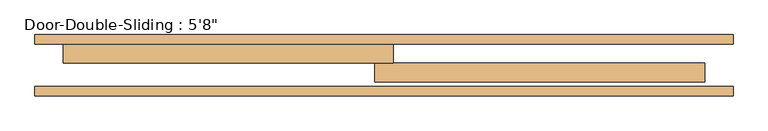
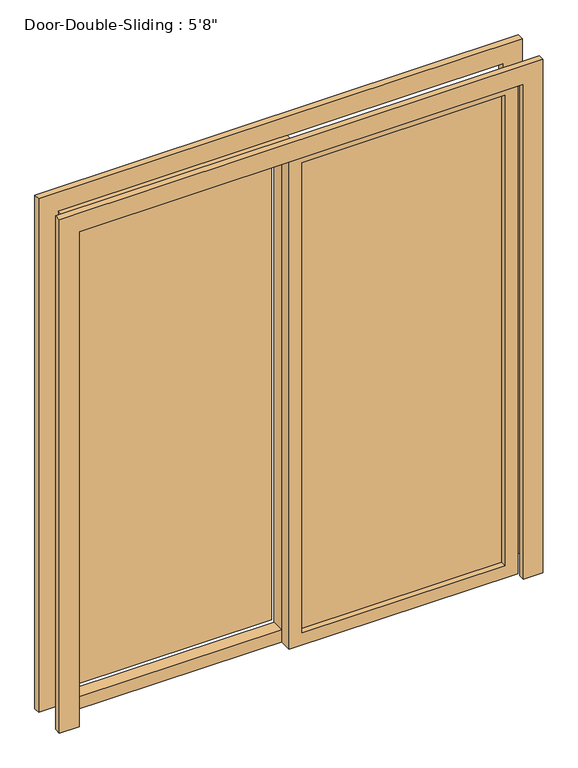
"""IFC4 building model written with IfcOpenShell, lengths in millimetres: door geometry."""

from ifc_helpers import new_model, si_unit, frame, origin, place, context, project, spatial, polyline, outline, extrude, source, transform, mapped, element, save


def door_c5e969d5(model_context):
    return source(origin(), model_context, "Body", "SweptSolid", [
        extrude(outline(polyline([(0.0, 939.8), (2108.2, 939.8), (2108.2, -939.8), (0.0, -939.8), (0.0, -863.6), (2032.0, -863.6), (2032.0, 863.6), (0.0, 863.6), (0.0, 939.8)])), frame((0.0, 184.15, 0.0), z_axis=(0.0, 1.0, 0.0), x_axis=(0.0, 0.0, 1.0)), (0.0, 0.0, 1.0), 25.4),
        extrude(outline(polyline([(0.0, -939.8), (0.0, -863.6), (2032.0, -863.6), (2032.0, 863.6), (0.0, 863.6), (0.0, 939.8), (2108.2, 939.8), (2108.2, -939.8), (0.0, -939.8)])), frame((0.0, 44.45, 0.0), z_axis=(0.0, 1.0, 0.0), x_axis=(0.0, 0.0, 1.0)), (0.0, 0.0, 1.0), 25.4),
        extrude(outline(polyline([(2032.0, 25.4), (2032.0, -863.6), (0.0, -863.6), (0.0, 25.4), (2032.0, 25.4)]), holes=[polyline([(1981.2, -25.4), (50.8, -25.4), (50.8, -812.8), (1981.2, -812.8), (1981.2, -25.4)])]), frame((0.0, 133.35, 0.0), z_axis=(0.0, 1.0, 0.0), x_axis=(0.0, 0.0, 1.0)), (0.0, 0.0, 1.0), 50.8),
        extrude(outline(polyline([(2032.0, -25.4), (0.0, -25.4), (0.0, 863.6), (2032.0, 863.6), (2032.0, -25.4)]), holes=[polyline([(1981.2, 25.4), (1981.2, 812.8), (50.8, 812.8), (50.8, 25.4), (1981.2, 25.4)])]), frame((0.0, 82.55, 0.0), z_axis=(0.0, 1.0, 0.0), x_axis=(0.0, 0.0, 1.0)), (0.0, 0.0, 1.0), 50.8),
        extrude(outline(polyline([(-25.4, 200.025), (-812.8, 200.025), (-812.8, 206.375), (-25.4, 206.375), (-25.4, 200.025)])), frame((0.0, 0.0, 50.8), z_axis=(0.0, 0.0, 1.0), x_axis=(1.0, 0.0, 0.0)), (0.0, 0.0, 1.0), 1930.4),
        extrude(outline(polyline([(25.4, 111.125), (812.8, 111.125), (812.8, 104.775), (25.4, 104.775), (25.4, 111.125)])), frame((0.0, 0.0, 50.8), z_axis=(0.0, 0.0, 1.0), x_axis=(1.0, 0.0, 0.0)), (0.0, 0.0, 1.0), 1930.4),
    ])


if __name__ == "__main__":
    model = new_model("IFC4")
    model_context = context("Model", 3, world=origin())
    ifc_project = project(units=[si_unit("LENGTHUNIT", "METRE", prefix="MILLI")], contexts=[model_context])
    site = spatial("IfcSite", under=ifc_project)
    building = spatial("IfcBuilding", under=site)
    placement = place(None, origin())
    door_shape = door_c5e969d5(model_context)
    element("IfcDoor", 1, ObjectType="Door-Double-Sliding : 5'8\"", at=placement, inside=building, context=model_context, shape_type="MappedRepresentation", body=[
        mapped(door_shape, transform((0.0, 0.0, 0.0), x_axis=(1.0, 0.0, 0.0), y_axis=(0.0, 1.0, 0.0), z_axis=(0.0, 0.0, 1.0))),
    ])
    save(model, "model.ifc")

# Revit data of these elements
# Type "Door-Double-Sliding : 5'8\""
#   Type Mark = "51"
#   Construction Type Id = "opn-d45"
#   Assembly Code = "C1020"
#   Analytic Construction = "Wood frame, double glass door "
#   Thickness = 0' - 2"
#   Thermal Resistance (R) = 0.31964 (m²·K)/W
#   Heat Transfer Coefficient (U) = 3.12872 W/(m²·K)
#   Height = 6' - 8"
#   Rail Width = 0' - 2"
#   Stiles = 0' - 2"
#   Trim Projection Ext = 0' - 1"
#   Trim Projection Int = 0' - 1"
#   Trim Width = 0' - 3"
#   Width = 5' - 8"
#   Define Thermal Properties by = 1
#   Glazing = Glass
#   Panel Material = Wood - Birch - Solid Stained Light Low Gloss
#   Trim Material = Paint - Sienna
#   Visual Light Transmittance = 0
#   Solar Heat Gain Coefficient = 0
#   Function = (empty or 0)
#   Wall Closure = (empty or 0)
# Element 1 (IfcDoor, "Door-Double-Sliding : 5'8\"")
#   Materials on its faces: "Paint - Sienna", "Wood - Birch - Solid Stained Light Low Gloss", "Glass"
# Materials
#   "Glass": class "Glass", colour RGB 0 128 192, transparency 0.9, Description = "Soda Lime Glass", Cost = 0
#   "Wood - Birch - Solid Stained Light Low Gloss": class "Wood", colour RGB 210 159 95, transparency 0, Cost = 0
#   "Paint - Sienna": colour RGB 118 70 51, transparency 0, Cost = 0
